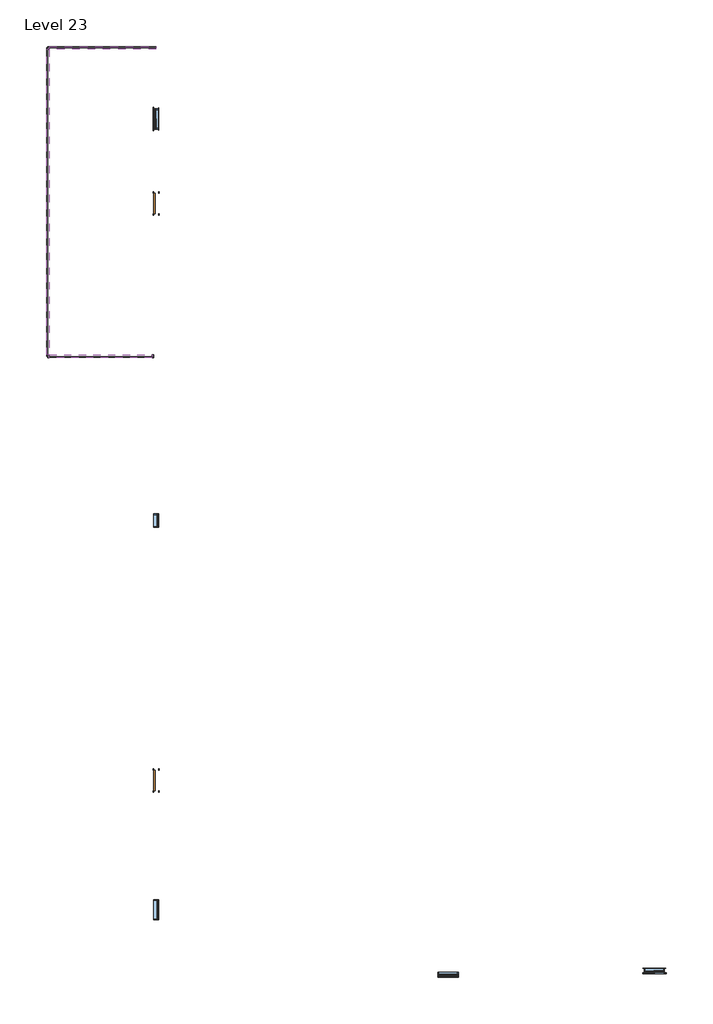
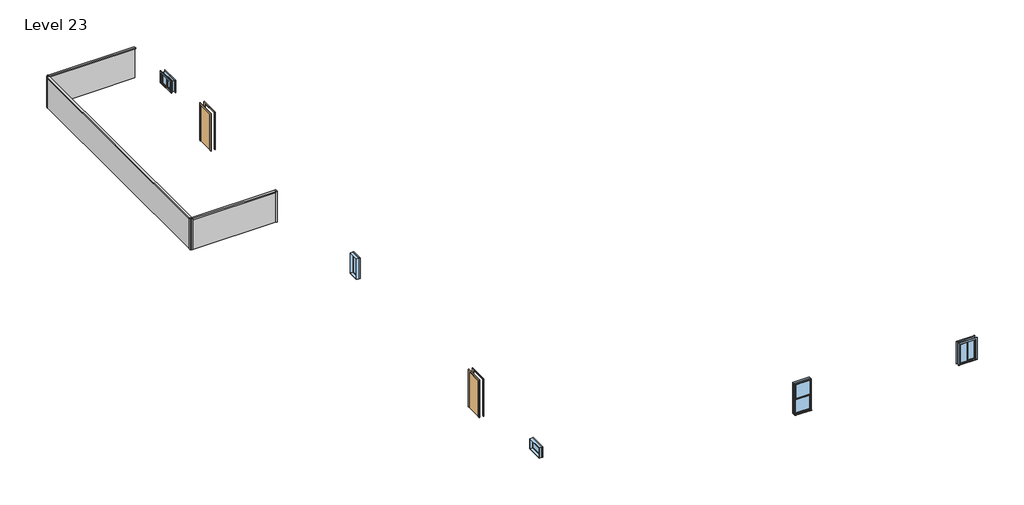
# One storey: 8 members, 5 windows, 3 plates, 2 doors.
"""IFC4 building model written with IfcOpenShell, lengths in millimetres."""

from ifc_helpers import new_model, si_unit, origin, place, context, project, spatial, transform, mapped, element, save
from components import door_54dd4da4, member_a0ba9e48, member_2fae0574, member_34ed8139, member_5c8c9790, system_panel_glazed_5a8eca4b, system_panel_glazed_372aa133, system_panel_glazed_ed669c81, window_f274a882, window_80bd9af0, window_57c3ee1c, window_a4355bb3, window_54100e87

model = new_model("IFC4")

# Units and contexts
model_context = context("Model", 3, world=origin())
ifc_project = project(units=[si_unit("LENGTHUNIT", "METRE", prefix="MILLI")], contexts=[model_context])

# Site, building, storey
site = spatial("IfcSite", under=ifc_project)
building = spatial("IfcBuilding", under=site)
storey = spatial("IfcBuildingStorey", under=building, Name="Level 23", Elevation=36576.0)

# Doors
placement = place(None, origin())
door_shape = door_54dd4da4(model_context)
element("IfcDoor", 1, ObjectType="Single-Flush : 36\" x 84\"", at=placement, inside=storey, context=model_context, shape_type="MappedRepresentation", body=[
    mapped(door_shape, transform((-15175.038074, 13799.8014639, 36576.0), x_axis=(0.0, 1.0, 0.0), y_axis=(-1.0, 0.0, 0.0), z_axis=(0.0, 0.0, 1.0))),
])
element("IfcDoor", 2, ObjectType="Single-Flush : 36\" x 84\"", at=placement, inside=storey, context=model_context, shape_type="MappedRepresentation", body=[
    mapped(door_shape, transform((-15175.038074, -12176.1915889, 36576.0), x_axis=(0.0, 1.0, 0.0), y_axis=(-1.0, 0.0, 0.0), z_axis=(0.0, 0.0, 1.0))),
])

# Members
member_shape = member_a0ba9e48(model_context)
element("IfcMember", 3, ObjectType="Rectangular Mullion : 2.5\" x 5\" rectangular", at=placement, inside=storey, context=model_context, shape_type="MappedRepresentation", body=[
    mapped(member_shape, transform((-15175.038074, 20810.2014639, 38100.0), x_axis=(0.0, 0.0, 1.0), y_axis=(0.0, -1.0, 0.0), z_axis=(1.0, 0.0, 0.0))),
])
member_2_shape = member_2fae0574(model_context)
element("IfcMember", 4, ObjectType="Rectangular Mullion : 2.5\" x 5\" rectangular", at=placement, inside=storey, context=model_context, shape_type="MappedRepresentation", body=[
    mapped(member_2_shape, transform((-20051.838074, 20810.2014639, 38100.0), x_axis=(-1.0, 0.0, 0.0), y_axis=(0.0, -1.0, 0.0), z_axis=(0.0, 0.0, 1.0))),
])
element("IfcMember", 5, ObjectType="Rectangular Mullion : 2.5\" x 5\" rectangular", at=placement, inside=storey, context=model_context, shape_type="MappedRepresentation", body=[
    mapped(member_2_shape, transform((-20051.838074, 6927.4727834, 38100.0), x_axis=(0.0, -1.0, 0.0), y_axis=(1.0, 0.0, 0.0), z_axis=(0.0, 0.0, 1.0))),
])
element("IfcMember", 6, ObjectType="Rectangular Mullion : 2.5\" x 5\" rectangular", at=placement, inside=storey, context=model_context, shape_type="MappedRepresentation", body=[
    mapped(member_2_shape, transform((-15295.688074, 6927.4727834, 38100.0), x_axis=(1.0, 0.0, 0.0), y_axis=(0.0, 1.0, 0.0), z_axis=(0.0, 0.0, 1.0))),
])
element("IfcMember", 7, ObjectType="Rectangular Mullion : 2.5\" x 5\" rectangular", at=placement, inside=storey, context=model_context, shape_type="MappedRepresentation", body=[
    mapped(member_2_shape, transform((-20051.838074, 6927.4727834, 36271.2), x_axis=(-1.0, 0.0, 0.0), y_axis=(0.0, 1.0, 0.0), z_axis=(0.0, 0.0, -1.0))),
])
element("IfcMember", 8, ObjectType="Rectangular Mullion : 2.5\" x 5\" rectangular", at=placement, inside=storey, context=model_context, shape_type="MappedRepresentation", body=[
    mapped(member_2_shape, transform((-20051.838074, 20810.2014639, 36271.2), x_axis=(0.0, 1.0, 0.0), y_axis=(1.0, 0.0, 0.0), z_axis=(0.0, 0.0, -1.0))),
])
member_3_shape = member_34ed8139(model_context)
element("IfcMember", 9, ObjectType="Rectangular Mullion : 2.5\" x 5\" rectangular", at=placement, inside=storey, context=model_context, shape_type="MappedRepresentation", body=[
    mapped(member_3_shape, transform((-20051.838074, 20746.7014639, 38100.0), x_axis=(0.0, 0.0, 1.0), y_axis=(1.0, 0.0, 0.0), z_axis=(0.0, 1.0, 0.0))),
])
member_4_shape = member_5c8c9790(model_context)
element("IfcMember", 10, ObjectType="Rectangular Mullion : 2.5\" x 5\" rectangular", at=placement, inside=storey, context=model_context, shape_type="MappedRepresentation", body=[
    mapped(member_4_shape, transform((-19988.338074, 6927.4727834, 38100.0), x_axis=(0.0, 0.0, 1.0), y_axis=(0.0, 1.0, 0.0), z_axis=(-1.0, 0.0, 0.0))),
])

# Plates
system_panel_glazed_shape = system_panel_glazed_5a8eca4b(model_context)
element("IfcPlate", 11, ObjectType="System Panel : Glazed", at=placement, inside=storey, context=model_context, shape_type="MappedRepresentation", body=[
    mapped(system_panel_glazed_shape, transform((-17581.688074, 20810.2014639, 36271.2), x_axis=(1.0, 0.0, 0.0), y_axis=(0.0, 1.0, 0.0), z_axis=(0.0, 0.0, 1.0))),
])
system_panel_glazed_2_shape = system_panel_glazed_372aa133(model_context)
element("IfcPlate", 12, ObjectType="System Panel : Glazed", at=placement, inside=storey, context=model_context, shape_type="MappedRepresentation", body=[
    mapped(system_panel_glazed_2_shape, transform((-20051.838074, 13868.8371237, 36271.2), x_axis=(0.0, 1.0, 0.0), y_axis=(-1.0, 0.0, 0.0), z_axis=(0.0, 0.0, 1.0))),
])
system_panel_glazed_3_shape = system_panel_glazed_ed669c81(model_context)
element("IfcPlate", 13, ObjectType="System Panel : Glazed", at=placement, inside=storey, context=model_context, shape_type="MappedRepresentation", body=[
    mapped(system_panel_glazed_3_shape, transform((-17673.763074, 6927.4727834, 36271.2), x_axis=(-1.0, 0.0, 0.0), y_axis=(0.0, -1.0, 0.0), z_axis=(0.0, 0.0, 1.0))),
])

# Windows
window_shape = window_f274a882(model_context)
element("IfcWindow", 14, ObjectType="Double Hung : 36\" x 72\"", at=placement, inside=storey, context=model_context, shape_type="MappedRepresentation", body=[
    mapped(window_shape, transform((-2017.838074, -20921.9985361, 36960.313115), x_axis=(-1.0, 0.0, 0.0), y_axis=(0.0, -1.0, 0.0), z_axis=(0.0, 0.0, 1.0))),
])
window_2_shape = window_80bd9af0(model_context)
element("IfcWindow", 15, ObjectType="Fixed : 24\" x 48\"", at=placement, inside=storey, context=model_context, shape_type="MappedRepresentation", body=[
    mapped(window_2_shape, transform((-15175.038074, -518.5213044, 36576.0), x_axis=(0.0, -1.0, 0.0), y_axis=(1.0, 0.0, 0.0), z_axis=(0.0, 0.0, 1.0))),
])
window_3_shape = window_57c3ee1c(model_context)
element("IfcWindow", 16, ObjectType="Fixed : 36\" x 24\"", at=placement, inside=storey, context=model_context, shape_type="MappedRepresentation", body=[
    mapped(window_3_shape, transform((-15175.038074, -18041.8099202, 36735.9868241), x_axis=(0.0, -1.0, 0.0), y_axis=(1.0, 0.0, 0.0), z_axis=(0.0, 0.0, 1.0))),
])
window_4_shape = window_a4355bb3(model_context)
element("IfcWindow", 17, ObjectType="Slider with Trim : 36\" x 24\"", at=placement, inside=storey, context=model_context, shape_type="MappedRepresentation", body=[
    mapped(window_4_shape, transform((-15175.038074, 17609.8014639, 36768.0078244), x_axis=(0.0, 1.0, 0.0), y_axis=(-1.0, 0.0, 0.0), z_axis=(0.0, 0.0, 1.0))),
])
window_5_shape = window_54100e87(model_context)
element("IfcWindow", 18, ObjectType="Slider with Trim : 36\" x 48\"", at=placement, inside=storey, context=model_context, shape_type="MappedRepresentation", body=[
    mapped(window_5_shape, transform((7278.561926, -20744.1985361, 35967.9341516), x_axis=(-1.0, 0.0, 0.0), y_axis=(0.0, -1.0, 0.0), z_axis=(0.0, 0.0, 1.0))),
])

save(model, "model.ifc")

# Revit data of these elements
# Type "Single-Flush : 36\" x 84\""
#   Type Mark = "1"
#   Construction Type Id = "MDOOR"
#   Assembly Code = "C1020"
#   Analytic Construction = "Metal"
#   Thickness = 0' - 2"
#   Heat Transfer Coefficient (U) = 0.651978 BTU/(h·ft²·°F)
#   Height = 7' - 0"
#   Trim Projection Ext = 0' - 1"
#   Trim Projection Int = 0' - 1"
#   Trim Width = 0' - 3"
#   Width = 3' - 0"
#   Define Thermal Properties by = 1
#   Door Material = Door - Panel
#   Frame Material = Door - Frame
#   Visual Light Transmittance = 0
#   Solar Heat Gain Coefficient = 0
#   Function = (empty or 0)
#   Wall Closure = (empty or 0)
# Type "Rectangular Mullion : 2.5\" x 5\" rectangular"
#   built-in parameter 1007304 = 0.416667 (stored number, unit not read)
#   built-in parameter 1007301 = 0.104167 (stored number, unit not read)
#   built-in parameter 1007300 = 0.104167 (stored number, unit not read)
# Type "System Panel : Glazed"
#   Construction Type Id = "GSP4R"
#   Analytic Construction = "1/8 in Pilkington single glazing"
#   Visual Light Transmittance = 0.9
#   Solar Heat Gain Coefficient = 0.86
#   Heat Transfer Coefficient (U) = 1.18115 BTU/(h·ft²·°F)
# Type "Double Hung : 36\" x 72\""
#   Type Mark = "18"
#   Construction Type Id = "GSP4R"
#   Assembly Code = "B2020100"
#   Analytic Construction = "1/8 in Pilkington single glazing"
#   Visual Light Transmittance = 0.9
#   Solar Heat Gain Coefficient = 0.78
#   Heat Transfer Coefficient (U) = 0.6496 BTU/(h·ft²·°F)
#   Height = 6' - 0"
#   Default Sill Height = 1' - 0"
#   Width = 3' - 0"
#   Window Inset = 0' - 0 3/4"
#   Define Thermal Properties by = 1
#   Glass Pane Material = Glass
#   Sash Material = Sash
#   Description = (empty or 0)
#   Wall Closure = (empty or 0)
# Type "Fixed : 24\" x 48\""
#   Type Mark = "2"
#   Construction Type Id = "GSP4R"
#   Assembly Code = "B2020100"
#   Analytic Construction = "1/8 in Pilkington single glazing"
#   Visual Light Transmittance = 0.9
#   Solar Heat Gain Coefficient = 0.78
#   Heat Transfer Coefficient (U) = 0.6496 BTU/(h·ft²·°F)
#   Height = 4' - 0"
#   Default Sill Height = 3' - 0"
#   Width = 2' - 0"
#   Window Inset = 0' - 0 3/4"
#   Define Thermal Properties by = 1
#   Glass Pane Material = Glass
#   Sash Material = Sash
#   Wall Closure = (empty or 0)
# Type "Fixed : 36\" x 24\""
#   Type Mark = "8"
#   Construction Type Id = "GSP4R"
#   Assembly Code = "B2020100"
#   Analytic Construction = "1/8 in Pilkington single glazing"
#   Visual Light Transmittance = 0.9
#   Solar Heat Gain Coefficient = 0.78
#   Heat Transfer Coefficient (U) = 0.6496 BTU/(h·ft²·°F)
#   Height = 2' - 0"
#   Default Sill Height = 3' - 0"
#   Width = 3' - 0"
#   Window Inset = 0' - 0 3/4"
#   Define Thermal Properties by = 1
#   Glass Pane Material = Glass
#   Sash Material = Sash
#   Wall Closure = (empty or 0)
# Type "Slider with Trim : 36\" x 24\""
#   Type Mark = "23"
#   Construction Type Id = "GSP4R"
#   Assembly Code = "B2020100"
#   Analytic Construction = "1/8 in Pilkington single glazing"
#   Visual Light Transmittance = 0.9
#   Solar Heat Gain Coefficient = 0.78
#   Heat Transfer Coefficient (U) = 0.6496 BTU/(h·ft²·°F)
#   Height = 2' - 0"
#   Default Sill Height = 3' - 0"
#   Trim Projection - Ext. = 0' - 0 3/4"
#   Trim Projection - Int. = 0' - 0 3/4"
#   Trim Width - Exterior = 0' - 3 1/2"
#   Trim Width - Interior = 0' - 3 1/2"
#   Width = 3' - 0"
#   Window Inset = 0' - 0 3/4"
#   Define Thermal Properties by = 1
#   Glass Pane Material = Glass
#   Sash Material = Sash
#   Trim Exterior Material = Trim
#   Trim Interior Material = Trim
#   Wall Closure = (empty or 0)
# Type "Slider with Trim : 36\" x 48\""
#   Type Mark = "22"
#   Construction Type Id = "GSP4R"
#   Assembly Code = "B2020100"
#   Analytic Construction = "1/8 in Pilkington single glazing"
#   Visual Light Transmittance = 0.9
#   Solar Heat Gain Coefficient = 0.78
#   Heat Transfer Coefficient (U) = 0.6496 BTU/(h·ft²·°F)
#   Height = 4' - 0"
#   Default Sill Height = 3' - 0"
#   Trim Projection - Ext. = 0' - 0 3/4"
#   Trim Projection - Int. = 0' - 0 3/4"
#   Trim Width - Exterior = 0' - 3 1/2"
#   Trim Width - Interior = 0' - 3 1/2"
#   Width = 3' - 0"
#   Window Inset = 0' - 0 3/4"
#   Define Thermal Properties by = 1
#   Glass Pane Material = Glass
#   Sash Material = Sash
#   Trim Exterior Material = Trim
#   Trim Interior Material = Trim
#   Wall Closure = (empty or 0)
# Elements 1, 2 (IfcDoor, "Single-Flush : 36\" x 84\"")
#   Phase Created = New Construction
#   Materials on its faces: "Door - Frame", "Door - Panel"
# Elements 3, 4, 5, 6, 7, 8, 9, 10 (IfcMember, "Rectangular Mullion : 2.5\" x 5\" rectangular")
#   Phase Created = New Construction
#   Materials on its faces: "Aluminum"
# Elements 11, 12, 13 (IfcPlate, "System Panel : Glazed")
#   Phase Created = New Construction
#   Materials on its faces: "Glass"
# Element 14 (IfcWindow, "Double Hung : 36\" x 72\"")
#   Mark = "1"
#   Phase Created = New Construction
#   Materials on its faces: "Sash", "Glass"
# Element 15 (IfcWindow, "Fixed : 24\" x 48\"")
#   Mark = "45"
#   Phase Created = New Construction
#   Materials on its faces: "Sash", "Glass"
# Element 16 (IfcWindow, "Fixed : 36\" x 24\"")
#   Mark = "67"
#   Phase Created = New Construction
#   Materials on its faces: "Sash", "Glass"
# Element 17 (IfcWindow, "Slider with Trim : 36\" x 24\"")
#   Mark = "56"
#   Phase Created = New Construction
#   Materials on its faces: "Sash", "Trim", "Glass"
# Element 18 (IfcWindow, "Slider with Trim : 36\" x 48\"")
#   Mark = "23"
#   Phase Created = New Construction
#   Materials on its faces: "Sash", "Trim", "Glass"
# Materials
#   "Door - Panel": class "Wood", colour RGB 210 159 95, transparency 0
#   "Door - Frame": colour RGB 118 70 51, transparency 0
#   "Glass": class "Glass", colour RGB 0 128 192, transparency 0.75, Description = "Soda Lime Glass", Cost = 0
#   "Sash": class "Wood", colour RGB 224 178 126, transparency 0
#   "Trim": class "Wood", colour RGB 224 178 126, transparency 0
#   "Aluminum": class "Metal", colour RGB 247 247 247, transparency 0, Description = "Aluminum 6061", Cost = 0
